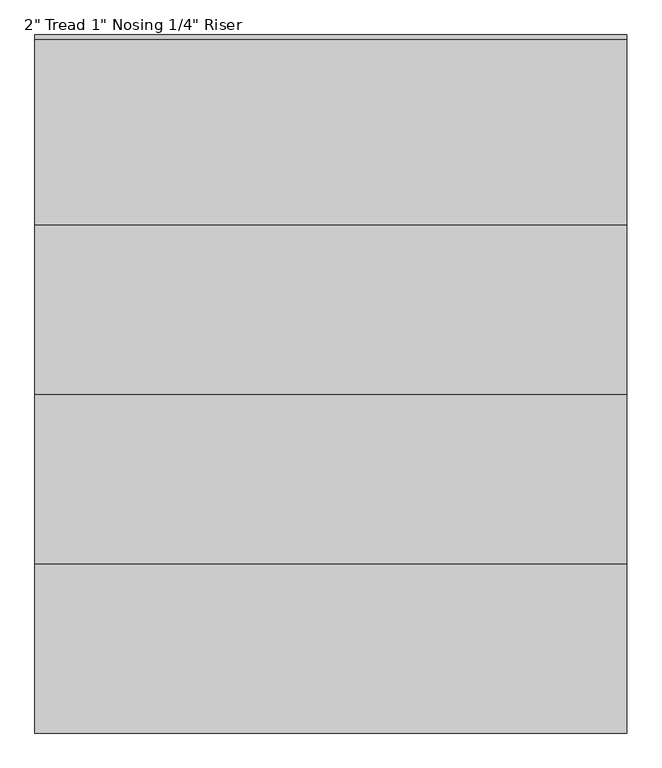
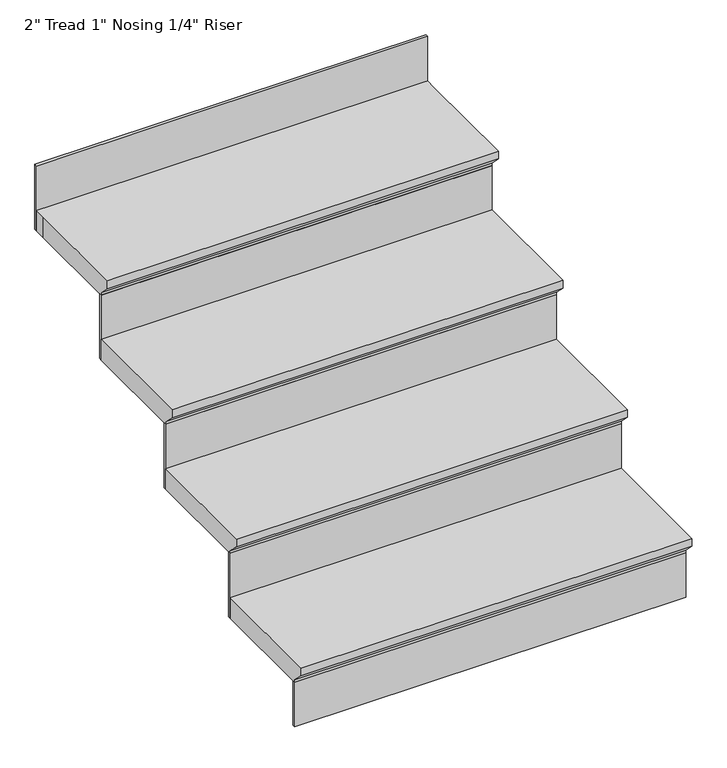
"""IFC4 building model written with IfcOpenShell, lengths in millimetres: stair flight geometry."""

from ifc_helpers import new_model, si_unit, origin, place, context, project, spatial, faceted_brep, source, transform, mapped, element, save


def stair_flight_8f72ff29(model_context):
    return source(origin(), model_context, "Body", "Brep", [
        faceted_brep([(-14090.1982861, 9720.1872586, 141.3710526), (-14090.1982861, 9720.1872586, 160.4210526), (-15004.5982861, 9720.1872586, 160.4210526), (-15004.5982861, 9720.1872586, 141.3710526), (-14090.1982861, 9745.5872586, 115.9710526), (-15004.5982861, 9745.5872586, 115.9710526), (-14090.1982861, 10007.2271024, 160.4210526), (-15004.5982861, 10007.2271024, 160.4210526), (-15004.5982861, 9745.5872586, 109.6210526), (-15004.5982861, 10007.2271024, 109.6210526), (-14090.1982861, 10007.2271024, 109.6210526), (-14090.1982861, 9745.5872586, 109.6210526)], [[[0, 1, 2, 3]], [[4, 0, 3, 5]], [[2, 1, 6, 7]], [[8, 9, 10, 11]], [[2, 7, 9, 8, 5, 3]], [[8, 11, 4, 5]], [[6, 1, 0, 4, 11, 10]], [[7, 6, 10, 9]]]),
        faceted_brep([(-14090.1982861, 9745.5872586, 109.6210526), (-14090.1982861, 9745.5872586, 0.0), (-14090.1982861, 9751.9372586, 0.0), (-14090.1982861, 9751.9372586, 109.6210526), (-15004.5982861, 9745.5872586, 109.6210526), (-15004.5982861, 9751.9372586, 109.6210526), (-15004.5982861, 9751.9372586, 0.0), (-15004.5982861, 9745.5872586, 0.0)], [[[0, 1, 2, 3]], [[4, 5, 6, 7]], [[1, 0, 4, 7]], [[2, 1, 7, 6]], [[3, 2, 6, 5]], [[0, 3, 5, 4]]]),
        faceted_brep([(-14090.1982861, 10007.2271024, 270.0421053), (-14090.1982861, 10007.2271024, 109.6210526), (-14090.1982861, 10013.5771024, 109.6210526), (-14090.1982861, 10013.5771024, 270.0421053), (-15004.5982861, 10007.2271024, 270.0421053), (-15004.5982861, 10013.5771024, 270.0421053), (-15004.5982861, 10013.5771024, 109.6210526), (-15004.5982861, 10007.2271024, 109.6210526)], [[[0, 1, 2, 3]], [[4, 5, 6, 7]], [[1, 0, 4, 7]], [[2, 1, 7, 6]], [[3, 2, 6, 5]], [[0, 3, 5, 4]]]),
        faceted_brep([(-15004.5982861, 9981.8271024, 320.8421053), (-14090.1982861, 9981.8271024, 320.8421053), (-14090.1982861, 10268.8669461, 320.8421053), (-15004.5982861, 10268.8669461, 320.8421053), (-15004.5982861, 10007.2271024, 270.0421053), (-15004.5982861, 10268.8669461, 270.0421053), (-14090.1982861, 10268.8669461, 270.0421053), (-14090.1982861, 10007.2271024, 270.0421053), (-15004.5982861, 10007.2271024, 276.3921053), (-15004.5982861, 9981.8271024, 301.7921053), (-14090.1982861, 10007.2271024, 276.3921053), (-14090.1982861, 9981.8271024, 301.7921053)], [[[0, 1, 2, 3]], [[4, 5, 6, 7]], [[0, 3, 5, 4, 8, 9]], [[4, 7, 10, 8]], [[2, 1, 11, 10, 7, 6]], [[3, 2, 6, 5]], [[11, 1, 0, 9]], [[10, 11, 9, 8]]]),
        faceted_brep([(-14090.1982861, 10268.8669461, 430.4631579), (-14090.1982861, 10268.8669461, 270.0421053), (-14090.1982861, 10275.2169461, 270.0421053), (-14090.1982861, 10275.2169461, 430.4631579), (-15004.5982861, 10268.8669461, 430.4631579), (-15004.5982861, 10275.2169461, 430.4631579), (-15004.5982861, 10275.2169461, 270.0421053), (-15004.5982861, 10268.8669461, 270.0421053)], [[[0, 1, 2, 3]], [[4, 5, 6, 7]], [[1, 0, 4, 7]], [[2, 1, 7, 6]], [[3, 2, 6, 5]], [[0, 3, 5, 4]]]),
        faceted_brep([(-15004.5982861, 10243.4669461, 481.2631579), (-14090.1982861, 10243.4669461, 481.2631579), (-14090.1982861, 10530.5067899, 481.2631579), (-15004.5982861, 10530.5067899, 481.2631579), (-15004.5982861, 10268.8669461, 430.4631579), (-15004.5982861, 10530.5067899, 430.4631579), (-14090.1982861, 10530.5067899, 430.4631579), (-14090.1982861, 10268.8669461, 430.4631579), (-15004.5982861, 10268.8669461, 436.8131579), (-15004.5982861, 10243.4669461, 462.2131579), (-14090.1982861, 10268.8669461, 436.8131579), (-14090.1982861, 10243.4669461, 462.2131579)], [[[0, 1, 2, 3]], [[4, 5, 6, 7]], [[0, 3, 5, 4, 8, 9]], [[4, 7, 10, 8]], [[2, 1, 11, 10, 7, 6]], [[3, 2, 6, 5]], [[11, 1, 0, 9]], [[10, 11, 9, 8]]]),
        faceted_brep([(-14090.1982861, 10792.1466336, 751.3052632), (-14090.1982861, 10792.1466336, 590.8842105), (-14090.1982861, 10798.4966336, 590.8842105), (-14090.1982861, 10798.4966336, 751.3052632), (-15004.5982861, 10792.1466336, 751.3052632), (-15004.5982861, 10798.4966336, 751.3052632), (-15004.5982861, 10798.4966336, 590.8842105), (-15004.5982861, 10792.1466336, 590.8842105)], [[[0, 1, 2, 3]], [[4, 5, 6, 7]], [[1, 0, 4, 7]], [[2, 1, 7, 6]], [[3, 2, 6, 5]], [[0, 3, 5, 4]]]),
        faceted_brep([(-14090.1982861, 10530.5067899, 590.8842105), (-14090.1982861, 10530.5067899, 430.4631579), (-14090.1982861, 10536.8567899, 430.4631579), (-14090.1982861, 10536.8567899, 590.8842105), (-15004.5982861, 10530.5067899, 590.8842105), (-15004.5982861, 10536.8567899, 590.8842105), (-15004.5982861, 10536.8567899, 430.4631579), (-15004.5982861, 10530.5067899, 430.4631579)], [[[0, 1, 2, 3]], [[4, 5, 6, 7]], [[1, 0, 4, 7]], [[2, 1, 7, 6]], [[3, 2, 6, 5]], [[0, 3, 5, 4]]]),
        faceted_brep([(-15004.5982861, 10792.1466336, 641.6842105), (-15004.5982861, 10766.7466336, 641.6842105), (-15004.5982861, 10505.1067899, 641.6842105), (-14090.1982861, 10505.1067899, 641.6842105), (-14090.1982861, 10766.7466336, 641.6842105), (-14090.1982861, 10792.1466336, 641.6842105), (-15004.5982861, 10766.7466336, 590.8842105), (-15004.5982861, 10792.1466336, 590.8842105), (-14090.1982861, 10792.1466336, 590.8842105), (-14090.1982861, 10766.7466336, 590.8842105), (-14090.1982861, 10530.5067899, 590.8842105), (-15004.5982861, 10530.5067899, 590.8842105), (-15004.5982861, 10530.5067899, 597.2342105), (-15004.5982861, 10505.1067899, 622.6342105), (-14090.1982861, 10530.5067899, 597.2342105), (-14090.1982861, 10505.1067899, 622.6342105)], [[[0, 1, 2, 3, 4, 5]], [[6, 7, 8, 9, 10, 11]], [[1, 0, 7, 6]], [[2, 1, 6, 11, 12, 13]], [[11, 10, 14, 12]], [[4, 3, 15, 14, 10, 9]], [[5, 4, 9, 8]], [[0, 5, 8, 7]], [[15, 3, 2, 13]], [[14, 15, 13, 12]]]),
    ])


if __name__ == "__main__":
    model = new_model("IFC4")
    model_context = context("Model", 3, world=origin())
    ifc_project = project(units=[si_unit("LENGTHUNIT", "METRE", prefix="MILLI")], contexts=[model_context])
    site = spatial("IfcSite", under=ifc_project)
    building = spatial("IfcBuilding", under=site)
    placement = place(None, origin())
    stair_flight_shape = stair_flight_8f72ff29(model_context)
    element("IfcStairFlight", 1, ObjectType="2\" Tread 1\" Nosing 1/4\" Riser", at=placement, inside=building, context=model_context, shape_type="MappedRepresentation", body=[
        mapped(stair_flight_shape, transform((0.0, 0.0, 0.0), x_axis=(1.0, 0.0, 0.0), y_axis=(0.0, 1.0, 0.0), z_axis=(0.0, 0.0, 1.0))),
    ])
    save(model, "model.ifc")
